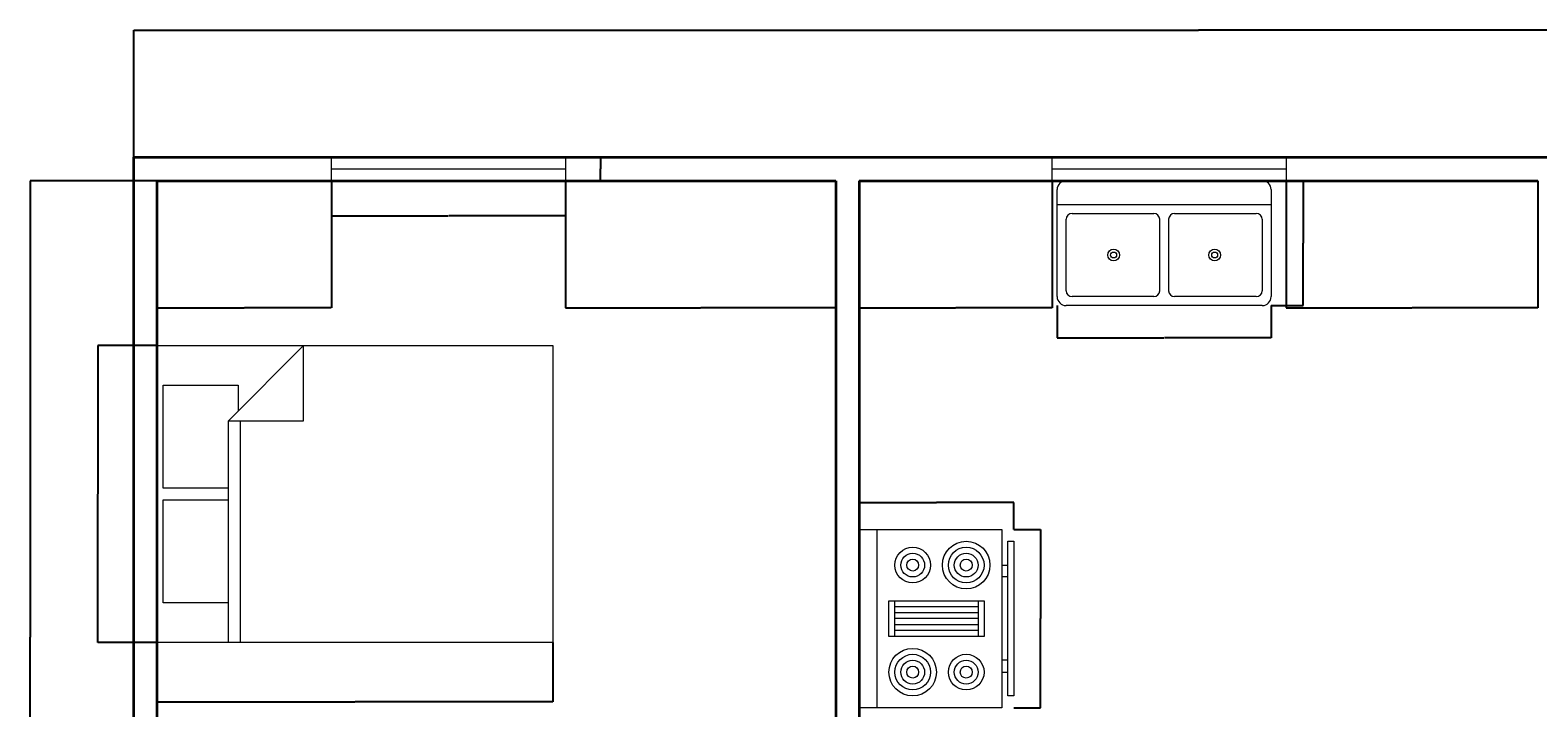
# Model space of a CAD drawing. Units: millimetres. Extents: x 1426 to 11512, y -8522 to 2664.
# Tile 3 of 4: x 1426 to 7869, y -230 to 2664. Entities that reach past the tile are written whole.
import ezdxf

# ---------------------------------------------------------------- set-up
doc = ezdxf.new("R2010")
doc.units = ezdxf.units.MM
for name, color, linetype, lineweight in [('A-ANNO-DIMS', 2, 'Continuous', 18), ('A-EQPM', 8, 'Continuous', 20), ('A-FLOR-FIXT', 9, 'Continuous', 20), ('A-FURN', 8, 'Continuous', 18), ('A-GLAZ', 4, 'Continuous', 18), ('A-WALL', 7, 'Continuous', 35)]:
    doc.layers.add(name, color=color, linetype=linetype, lineweight=lineweight)
doc.styles.get("Standard").update_dxf_attribs({"font": 'arial.ttf'})
doc.dimstyles.get("Standard").update_dxf_attribs({"dimtxt": 0.18, "dimasz": 0.18, "dimexe": 0.18, "dimexo": 0.0625, "dimgap": 0.09, "dimtad": 0, "dimtih": 1, "dimtoh": 1, "dimdec": 4, "dimzin": 0, "dimdsep": 46, "dimtxsty": 'Standard', "dimcen": 0.09, "dimadec": 0, "dimazin": 0, "dimtfac": 1, "dimtdec": 4, "dimtofl": 0, "dimtmove": 0, "dimatfit": 3, "dimfxl": 1, "dimtolj": 1, "dimtzin": 0, "dimarcsym": 0})

# ---------------------------------------------------------------- blocks, each defined once
blk = doc.blocks.new('Range-Oven - 30 in top')
for p, q in [((0, -3), (30, -3)), ((12, -6), (18, -6)), ((13, -20), (13, -6)), ((14, -6), (14, -20)), ((15, -20), (15, -6)), ((16, -6), (16, -20)), ((17, -20), (17, -6)), ((18, -20), (12, -20)), ((6, -24), (6, -25)), ((8, -25), (8, -24)), ((22, -25), (22, -24)), ((24, -24), (24, -25))]:
    blk.add_line(p, q)
for points in [[(0, -24), (0, 0), (30, 0), (30, -24)], [(12, -21), (12, -5), (18, -5), (18, -21)], [(2, -26), (2, -25), (28, -25), (28, -26)]]:
    blk.add_lwpolyline(points, close=True)
for centre, radius in [((6, -9), 4), ((6, -9), 3), ((6, -9), 2), ((24, -9), 3), ((24, -9), 2), ((6, -9), 1), ((24, -9), 1), ((6, -18), 3), ((24, -18), 4), ((24, -18), 3), ((6, -18), 2), ((6, -18), 1), ((24, -18), 2), ((24, -18), 1)]:
    blk.add_circle(centre, radius)
blk = doc.blocks.new('Sink-double - 36 in top')
for p, q in [((-18, -4), (18, -4)), ((-0.75, -18.5), (-0.75, -6.5)), ((0.75, -6.5), (0.75, -18.5))]:
    blk.add_line(p, q)
for points in [[(-16.5, 0), (16.5, 0)], [(-18, -19.5), (-18, -1.5)], [(18, -1.5), (18, -19.5)], [(-16.5, -18.5), (-16.5, -6.5)], [(-15.5, -5.5), (-1.75, -5.5)], [(1.75, -5.5), (15.5, -5.5)], [(16.5, -6.5), (16.5, -18.5)], [(-1.75, -19.5), (-15.5, -19.5)], [(15.5, -19.5), (1.75, -19.5)], [(16.5, -21), (-16.5, -21)]]:
    blk.add_lwpolyline(points)
for centre, radius in [((-8.5, -12.5), 1), ((-8.5, -12.5), 0.5), ((8.5, -12.5), 1), ((8.5, -12.5), 0.5)]:
    blk.add_circle(centre, radius)
for centre, radius, start, end in [((-16.5, -1.5), 1.5, 90, 180), ((16.5, -1.5), 1.5, 0, 90), ((-15.5, -6.5), 1, 90, 180), ((-1.75, -6.5), 1, 0, 90), ((1.75, -6.5), 1, 90, 180), ((15.5, -6.5), 1, 0, 90), ((-16.5, -19.5), 1.5, 180, 270), ((-15.5, -18.5), 1, 180, 270), ((-1.75, -18.5), 1, 270, 0), ((1.75, -18.5), 1, 180, 270), ((15.5, -18.5), 1, 270, 0), ((16.5, -19.5), 1.5, 270, 0)]:
    blk.add_arc(centre, radius, start, end)
blk = doc.blocks.new('Bed - Queen')
for p, q in [((0, -80.00003), (0, 0)), ((0, 0), (59.99999, 0)), ((59.99999, 0), (59.99999, -80.00003)), ((7.99999, -1.2), (28.79998, -1.2)), ((7.99999, -14.4), (7.99999, -1.2)), ((28.79998, -1.2), (28.79998, -14.4)), ((31.19999, -1.2), (51.99999, -1.2)), ((31.19999, -14.4), (31.19999, -1.2)), ((51.99999, -1.2), (51.99999, -16.4)), ((0, -14.4), (44.8, -14.4)), ((59.99999, -29.6), (44.8, -14.4)), ((44.8, -14.4), (44.8, -29.6)), ((44.8, -16.8), (0, -16.8)), ((51.99999, -16.4), (46.79936, -16.4)), ((44.8, -29.6), (59.99999, -29.6)), ((59.99999, -80.00003), (0, -80.00003))]:
    blk.add_line(p, q)
blk = doc.blocks.new('WIN-1000')
for p, q in [((0, 100), (1000, 100)), ((0, 0), (0, 100)), ((1000, 100), (1000, 0)), ((0, 50), (1000, 50)), ((1000, 0), (0, 0))]:
    blk.add_line(p, q)
blk = doc.blocks.new('*D14')
at = {"layer": 'A-ANNO-DIMS', "color": 0, "lineweight": -2, "transparency": 16777216}
for p, q in [((2713.3, 2020.9), (2713.3, 1870.8)), ((3713.3, 2020.9), (3713.3, 1870.8)), ((2713.5, 1870.9), (3212.1, 1870.9)), ((3713.1, 1870.9), (3214.6, 1870.9))]:
    blk.add_line(p, q, dxfattribs=at)
at = {"layer": 'A-ANNO-DIMS', "color": 0, "transparency": 16777216}
for points in [[(2713.5, 1871), (2713.5, 1870.9), (2713.3, 1870.9)], [(3713.1, 1871), (3713.1, 1870.9), (3713.3, 1870.9)]]:
    blk.add_solid(points, dxfattribs=at)
at = {"layer": 'Defpoints', "color": 0, "transparency": 16777216}
for p in [(2713.3, 2020.9), (3713.3, 2020.9), (3713.3, 1870.9)]:
    blk.add_point(p, dxfattribs=at)
at = {"layer": 'A-ANNO-DIMS', "color": 0, "transparency": 16777216, "insert": (3213.3, 1870.9), "char_height": 0.18, "attachment_point": 5}
blk.add_mtext('\\A1;WINDOW 1000 TYP.', dxfattribs=at)
blk = doc.blocks.new('*D15')
at = {"layer": 'A-ANNO-DIMS', "color": 0, "lineweight": -2, "transparency": 16777216}
for p, q in [((3713.4, 2120.9), (3863.5, 2120.9)), ((3863.3, 2120.8), (3863.3, 2071.1)), ((3863.3, 2021.1), (3863.3, 2070.8)), ((3713.4, 2020.9), (3863.5, 2020.9))]:
    blk.add_line(p, q, dxfattribs=at)
at = {"layer": 'A-ANNO-DIMS', "color": 0, "transparency": 16777216}
for points in [[(3863.3, 2120.8), (3863.3, 2120.8), (3863.3, 2120.9)], [(3863.3, 2021.1), (3863.3, 2021.1), (3863.3, 2020.9)]]:
    blk.add_solid(points, dxfattribs=at)
at = {"layer": 'Defpoints', "color": 0, "transparency": 16777216}
for p in [(3713.3, 2120.9), (3863.3, 2120.9), (3713.3, 2020.9)]:
    blk.add_point(p, dxfattribs=at)
at = {"layer": 'A-ANNO-DIMS', "color": 0, "transparency": 16777216, "insert": (3863.3, 2070.9), "char_height": 0.18, "attachment_point": 5}
blk.add_mtext('\\A1;100 TYP.', dxfattribs=at)
blk = doc.blocks.new('*D22')
at = {"layer": 'A-ANNO-DIMS', "color": 0, "lineweight": -2, "transparency": 16777216}
for p, q in [((1968.9, 49), (1968.9, -204.6)), ((3659.2, 49), (3659.2, -204.6)), ((1969.1, -204.5), (2813.4, -204.5)), ((3659, -204.5), (2814.7, -204.5))]:
    blk.add_line(p, q, dxfattribs=at)
at = {"layer": 'A-ANNO-DIMS', "color": 0, "transparency": 16777216}
for points in [[(1969.1, -204.4), (1969.1, -204.5), (1968.9, -204.5)], [(3659, -204.4), (3659, -204.5), (3659.2, -204.5)]]:
    blk.add_solid(points, dxfattribs=at)
at = {"layer": 'Defpoints', "color": 0, "transparency": 16777216}
for p in [(1968.9, 49.1), (3659.2, 49.1), (1968.9, -204.5)]:
    blk.add_point(p, dxfattribs=at)
at = {"layer": 'A-ANNO-DIMS', "color": 0, "transparency": 16777216, "insert": (2814, -204.5), "char_height": 0.18, "attachment_point": 5}
blk.add_mtext('\\A1;BED 1690', dxfattribs=at)
blk = doc.blocks.new('*D23')
at = {"layer": 'A-ANNO-DIMS', "color": 0, "lineweight": -2, "transparency": 16777216}
for p, q in [((1968.8, 1316.9), (1715.1, 1316.9)), ((1715.3, 1316.7), (1715.3, 683.2)), ((1715.3, 49.3), (1715.3, 682.8)), ((1968.8, 49.1), (1715.1, 49.1))]:
    blk.add_line(p, q, dxfattribs=at)
at = {"layer": 'A-ANNO-DIMS', "color": 0, "transparency": 16777216}
for points in [[(1715.3, 1316.7), (1715.3, 1316.7), (1715.3, 1316.9)], [(1715.3, 49.3), (1715.3, 49.3), (1715.3, 49.1)]]:
    blk.add_solid(points, dxfattribs=at)
at = {"layer": 'Defpoints', "color": 0, "transparency": 16777216}
for p in [(1715.3, 1316.9), (1968.9, 1316.9), (1968.9, 49.1)]:
    blk.add_point(p, dxfattribs=at)
at = {"layer": 'A-ANNO-DIMS', "color": 0, "transparency": 16777216, "insert": (1715.3, 683), "char_height": 0.18, "attachment_point": 5}
blk.add_mtext('\\A1;1268', dxfattribs=at)
blk = doc.blocks.new('*D28')
at = {"layer": 'A-ANNO-DIMS', "color": 0, "lineweight": -2, "transparency": 16777216}
for p, q in [((5629.3, 531.7), (5743.8, 531.7)), ((5743.6, 531.5), (5743.6, 150.9)), ((5743.6, -230.1), (5743.6, 150.5)), ((5629.3, -230.3), (5743.8, -230.3))]:
    blk.add_line(p, q, dxfattribs=at)
at = {"layer": 'A-ANNO-DIMS', "color": 0, "transparency": 16777216}
for points in [[(5743.5, 531.5), (5743.6, 531.5), (5743.6, 531.7)], [(5743.5, -230.1), (5743.6, -230.1), (5743.6, -230.3)]]:
    blk.add_solid(points, dxfattribs=at)
at = {"layer": 'Defpoints', "color": 0, "transparency": 16777216}
for p in [(5629.3, 531.7), (5743.6, 531.7), (5629.3, -230.3)]:
    blk.add_point(p, dxfattribs=at)
at = {"layer": 'A-ANNO-DIMS', "color": 0, "transparency": 16777216, "insert": (5743.6, 150.7), "char_height": 0.18, "attachment_point": 5}
blk.add_mtext('\\A1;RANGE 762', dxfattribs=at)
blk = doc.blocks.new('*D29')
at = {"layer": 'A-ANNO-DIMS', "color": 0, "lineweight": -2, "transparency": 16777216}
for p, q in [((4968.9, 531.8), (4968.9, 646.2)), ((4969.1, 646), (5298.8, 646)), ((5629.1, 646), (5299.4, 646)), ((5629.3, 531.8), (5629.3, 646.2))]:
    blk.add_line(p, q, dxfattribs=at)
at = {"layer": 'A-ANNO-DIMS', "color": 0, "transparency": 16777216}
for points in [[(4969.1, 646), (4969.1, 646), (4968.9, 646)], [(5629.1, 646), (5629.1, 646), (5629.3, 646)]]:
    blk.add_solid(points, dxfattribs=at)
at = {"layer": 'Defpoints', "color": 0, "transparency": 16777216}
for p in [(4968.9, 646), (4968.9, 531.7), (5629.3, 531.7)]:
    blk.add_point(p, dxfattribs=at)
at = {"layer": 'A-ANNO-DIMS', "color": 0, "transparency": 16777216, "insert": (5299.1, 646), "char_height": 0.18, "attachment_point": 5}
blk.add_mtext('\\A1;660', dxfattribs=at)
blk = doc.blocks.new('*D30')
at = {"layer": 'A-ANNO-DIMS', "color": 0, "lineweight": -2, "transparency": 16777216}
for p, q in [((5814.7, 1487.5), (5814.7, 1350.2)), ((6729.1, 1487.5), (6729.1, 1350.2)), ((5814.9, 1350.4), (6270.7, 1350.4)), ((6729, 1350.4), (6273.1, 1350.4))]:
    blk.add_line(p, q, dxfattribs=at)
at = {"layer": 'A-ANNO-DIMS', "color": 0, "transparency": 16777216}
for points in [[(5814.9, 1350.4), (5814.9, 1350.4), (5814.7, 1350.4)], [(6729, 1350.4), (6729, 1350.4), (6729.1, 1350.4)]]:
    blk.add_solid(points, dxfattribs=at)
at = {"layer": 'Defpoints', "color": 0, "transparency": 16777216}
for p in [(5814.7, 1487.5), (6729.1, 1487.5), (6729.1, 1350.4)]:
    blk.add_point(p, dxfattribs=at)
at = {"layer": 'A-ANNO-DIMS', "color": 0, "transparency": 16777216, "insert": (6271.9, 1350.4), "char_height": 0.18, "attachment_point": 5}
blk.add_mtext('\\A1;KITCHEN SINK 914', dxfattribs=at)
blk = doc.blocks.new('*D31')
at = {"layer": 'A-ANNO-DIMS', "color": 0, "lineweight": -2, "transparency": 16777216}
for p, q in [((6729.2, 2020.9), (6866.5, 2020.9)), ((6866.3, 2020.8), (6866.3, 1754.4)), ((6866.3, 1487.7), (6866.3, 1754.1)), ((6729.2, 1487.5), (6866.5, 1487.5))]:
    blk.add_line(p, q, dxfattribs=at)
at = {"layer": 'A-ANNO-DIMS', "color": 0, "transparency": 16777216}
for points in [[(6866.3, 2020.8), (6866.3, 2020.8), (6866.3, 2020.9)], [(6866.3, 1487.7), (6866.3, 1487.7), (6866.3, 1487.5)]]:
    blk.add_solid(points, dxfattribs=at)
at = {"layer": 'Defpoints', "color": 0, "transparency": 16777216}
for p in [(6729.1, 2020.9), (6866.3, 2020.9), (6729.1, 1487.5)]:
    blk.add_point(p, dxfattribs=at)
at = {"layer": 'A-ANNO-DIMS', "color": 0, "transparency": 16777216, "insert": (6866.3, 1754.2), "char_height": 0.18, "attachment_point": 5}
blk.add_mtext('\\A1;533', dxfattribs=at)
blk = doc.blocks.new('*D39')
at = {"layer": 'A-ANNO-DIMS', "color": 0, "lineweight": -2, "transparency": 16777216}
for p, q in [((1868.9, 2121), (1868.9, 2663.6)), ((1869.1, 2663.4), (6418.5, 2663.4)), ((10968.7, 2663.4), (6419.2, 2663.4)), ((10968.9, 2121), (10968.9, 2663.6))]:
    blk.add_line(p, q, dxfattribs=at)
at = {"layer": 'A-ANNO-DIMS', "color": 0, "transparency": 16777216}
for points in [[(1869.1, 2663.5), (1869.1, 2663.4), (1868.9, 2663.4)], [(10968.7, 2663.5), (10968.7, 2663.4), (10968.9, 2663.4)]]:
    blk.add_solid(points, dxfattribs=at)
at = {"layer": 'Defpoints', "color": 0, "transparency": 16777216}
for p in [(10968.9, 2663.4), (1868.9, 2120.9), (10968.9, 2120.9)]:
    blk.add_point(p, dxfattribs=at)
at = {"layer": 'A-ANNO-DIMS', "color": 0, "transparency": 16777216, "insert": (6418.9, 2663.4), "char_height": 0.18, "attachment_point": 5}
blk.add_mtext('\\A1;9100', dxfattribs=at)
blk = doc.blocks.new('*D43')
at = {"layer": 'A-ANNO-DIMS', "color": 0, "lineweight": -2, "transparency": 16777216}
for p, q in [((1968.8, 2020.9), (1426.2, 2020.9)), ((1426.4, 2020.8), (1426.4, 71.1)), ((1426.4, -1878.9), (1426.4, 70.8)), ((1968.8, -1879.1), (1426.2, -1879.1))]:
    blk.add_line(p, q, dxfattribs=at)
at = {"layer": 'A-ANNO-DIMS', "color": 0, "transparency": 16777216}
for points in [[(1426.3, 2020.8), (1426.4, 2020.8), (1426.4, 2020.9)], [(1426.3, -1878.9), (1426.4, -1878.9), (1426.4, -1879.1)]]:
    blk.add_solid(points, dxfattribs=at)
at = {"layer": 'Defpoints', "color": 0, "transparency": 16777216}
for p in [(1426.4, 2020.9), (1968.9, 2020.9), (1968.9, -1879.1)]:
    blk.add_point(p, dxfattribs=at)
at = {"layer": 'A-ANNO-DIMS', "color": 0, "transparency": 16777216, "insert": (1426.4, 70.9), "char_height": 0.18, "attachment_point": 5}
blk.add_mtext('\\A1;3900', dxfattribs=at)
blk = doc.blocks.new('*D54')
at = {"layer": 'A-ANNO-DIMS', "color": 0, "lineweight": -2, "transparency": 16777216}
for p, q in [((1968.9, 2020.9), (1968.9, 1478.3)), ((2713.3, 2020.9), (2713.3, 1478.3)), ((1969.1, 1478.4), (2340.7, 1478.4)), ((2713.1, 1478.4), (2341.5, 1478.4))]:
    blk.add_line(p, q, dxfattribs=at)
at = {"layer": 'A-ANNO-DIMS', "color": 0, "transparency": 16777216}
for points in [[(1969.1, 1478.5), (1969.1, 1478.4), (1968.9, 1478.4)], [(2713.1, 1478.5), (2713.1, 1478.4), (2713.3, 1478.4)]]:
    blk.add_solid(points, dxfattribs=at)
at = {"layer": 'Defpoints', "color": 0, "transparency": 16777216}
for p in [(1968.9, 2020.9), (2713.3, 2020.9), (1968.9, 1478.4)]:
    blk.add_point(p, dxfattribs=at)
at = {"layer": 'A-ANNO-DIMS', "color": 0, "transparency": 16777216, "insert": (2341.1, 1478.4), "char_height": 0.18, "attachment_point": 5}
blk.add_mtext('\\A1;744.4', dxfattribs=at)
blk = doc.blocks.new('*D55')
at = {"layer": 'A-ANNO-DIMS', "color": 0, "lineweight": -2, "transparency": 16777216}
for p, q in [((3713.3, 2020.9), (3713.3, 1478.3)), ((4868.9, 2020.9), (4868.9, 1478.3)), ((3713.5, 1478.4), (4290.6, 1478.4)), ((4868.7, 1478.4), (4291.5, 1478.4))]:
    blk.add_line(p, q, dxfattribs=at)
at = {"layer": 'A-ANNO-DIMS', "color": 0, "transparency": 16777216}
for points in [[(3713.5, 1478.5), (3713.5, 1478.4), (3713.3, 1478.4)], [(4868.7, 1478.5), (4868.7, 1478.4), (4868.9, 1478.4)]]:
    blk.add_solid(points, dxfattribs=at)
at = {"layer": 'Defpoints', "color": 0, "transparency": 16777216}
for p in [(3713.3, 2020.9), (4868.9, 2020.9), (3713.3, 1478.4)]:
    blk.add_point(p, dxfattribs=at)
at = {"layer": 'A-ANNO-DIMS', "color": 0, "transparency": 16777216, "insert": (4291.1, 1478.4), "char_height": 0.18, "attachment_point": 5}
blk.add_mtext('\\A1;1155.6', dxfattribs=at)
blk = doc.blocks.new('*D56')
at = {"layer": 'A-ANNO-DIMS', "color": 0, "lineweight": -2, "transparency": 16777216}
for p, q in [((4968.9, 2020.9), (4968.9, 1478.3)), ((5793.2, 2020.9), (5793.2, 1478.3)), ((4969.1, 1478.4), (5380.6, 1478.4)), ((5793, 1478.4), (5381.4, 1478.4))]:
    blk.add_line(p, q, dxfattribs=at)
at = {"layer": 'A-ANNO-DIMS', "color": 0, "transparency": 16777216}
for points in [[(4969.1, 1478.5), (4969.1, 1478.4), (4968.9, 1478.4)], [(5793, 1478.5), (5793, 1478.4), (5793.2, 1478.4)]]:
    blk.add_solid(points, dxfattribs=at)
at = {"layer": 'Defpoints', "color": 0, "transparency": 16777216}
for p in [(4968.9, 2020.9), (5793.2, 2020.9), (4968.9, 1478.4)]:
    blk.add_point(p, dxfattribs=at)
at = {"layer": 'A-ANNO-DIMS', "color": 0, "transparency": 16777216, "insert": (5381, 1478.4), "char_height": 0.18, "attachment_point": 5}
blk.add_mtext('\\A1;824.3', dxfattribs=at)
blk = doc.blocks.new('*D57')
at = {"layer": 'A-ANNO-DIMS', "color": 0, "lineweight": -2, "transparency": 16777216}
for p, q in [((6793.2, 2020.9), (6793.2, 1478.3)), ((7868.9, 2020.9), (7868.9, 1478.3)), ((6793.4, 1478.4), (7330.6, 1478.4)), ((7868.7, 1478.4), (7331.5, 1478.4))]:
    blk.add_line(p, q, dxfattribs=at)
at = {"layer": 'A-ANNO-DIMS', "color": 0, "transparency": 16777216}
for points in [[(6793.4, 1478.5), (6793.4, 1478.4), (6793.2, 1478.4)], [(7868.7, 1478.5), (7868.7, 1478.4), (7868.9, 1478.4)]]:
    blk.add_solid(points, dxfattribs=at)
at = {"layer": 'Defpoints', "color": 0, "transparency": 16777216}
for p in [(6793.2, 2020.9), (7868.9, 2020.9), (6793.2, 1478.4)]:
    blk.add_point(p, dxfattribs=at)
at = {"layer": 'A-ANNO-DIMS', "color": 0, "transparency": 16777216, "insert": (7331, 1478.4), "char_height": 0.18, "attachment_point": 5}
blk.add_mtext('\\A1;1075.7', dxfattribs=at)

msp = doc.modelspace()

# ---------------------------------------------------------------- linework, layer by layer
at = {"layer": 'A-WALL'}
for p, q in [((1868.87, 2120.94), (8976.97, 2120.94)), ((1868.87, -7979.06), (1868.87, 2120.94)), ((1968.87, 2020.94), (4868.87, 2020.94)), ((1968.87, -1879.06), (1968.87, 2020.94)), ((4868.87, 2020.94), (4868.87, -1879.06)), ((4968.87, 2020.94), (4968.87, -1879.06)), ((4968.87, 2020.94), (7868.87, 2020.94))]:
    msp.add_line(p, q, dxfattribs=at)

# ---------------------------------------------------------------- block references
at = {"layer": 'A-EQPM', "xscale": 25.4, "yscale": 25.4, "zscale": 25.4, "rotation": 90}
msp.add_blockref('Range-Oven - 30 in top', (4968.87, -230.3), dxfattribs=at)
at = {"layer": 'A-FLOR-FIXT', "xscale": 25.4, "yscale": 25.4, "zscale": 25.4}
msp.add_blockref('Sink-double - 36 in top', (6271.93, 2020.94), dxfattribs=at)
at = {"layer": 'A-FURN', "xscale": 21.12936966835213, "yscale": 21.12936966835213, "zscale": 21.12936966835213, "rotation": 89.99999999999999}
msp.add_blockref('Bed - Queen', (1968.87, 49.09), dxfattribs=at)
at = {"layer": 'A-GLAZ'}
for p in [(2713.31, 2020.94), (5793.19, 2020.94)]:
    msp.add_blockref('WIN-1000', p, dxfattribs=at)

# ---------------------------------------------------------------- dimensions: what is measured, and where the dimension line sits
at = {"layer": 'A-ANNO-DIMS'}
dim = msp.add_linear_dim(base=(10968.87, 2663.44), p1=(1868.87, 2120.94), p2=(10968.87, 2120.94), dimstyle='Standard', override={"dimdec": 0, "dimlfac": 1, "dimrnd": 0, "dimzin": 0, "dimdsep": 46, "dimlunit": 2}, dxfattribs=at)
dim.commit()
dim.dimension.update_dxf_attribs({"geometry": '*D39', "text_midpoint": (6418.87, 2663.44)})
for base, p1, p2, angle, text, picture, middle in [((3863.31, 2120.94), (3713.31, 2020.94), (3713.31, 2120.94), 90, '<> TYP.', '*D15', (3863.31, 2070.94)), ((5743.57, 531.7), (5629.27, -230.3), (5629.27, 531.7), 90, 'RANGE <>', '*D28', (5743.57, 150.7)), ((1968.87, -204.46), (3659.22, 49.09), (1968.87, 49.09), 180, 'BED <>', '*D22', (2814.05, -204.46))]:
    dim = msp.add_linear_dim(base=base, p1=p1, p2=p2, angle=angle, text=text, dimstyle='Standard', override={"dimdec": 0, "dimlfac": 1, "dimrnd": 0, "dimzin": 0, "dimdsep": 46, "dimlunit": 2}, dxfattribs=at)
    dim.commit()
    dim.dimension.update_dxf_attribs({"geometry": picture, "text_midpoint": middle})
for base, p1, p2, angle, override, picture, middle in [((1426.37, 2020.94), (1968.87, -1879.06), (1968.87, 2020.94), 90, {"dimdec": 0, "dimlfac": 1, "dimrnd": 0, "dimzin": 0, "dimdsep": 46, "dimlunit": 2}, '*D43', (1426.37, 70.94)), ((1968.87, 1478.44), (2713.31, 2020.94), (1968.87, 2020.94), 180, {"dimdec": 1, "dimlfac": 1, "dimrnd": 0, "dimzin": 0, "dimdsep": 46, "dimlunit": 2}, '*D54', (2341.09, 1478.44)), ((3713.31, 1478.44), (4868.87, 2020.94), (3713.31, 2020.94), 180, {"dimdec": 1, "dimlfac": 1, "dimrnd": 0, "dimzin": 0, "dimdsep": 46, "dimlunit": 2}, '*D55', (4291.09, 1478.44)), ((4968.87, 1478.44), (5793.19, 2020.94), (4968.87, 2020.94), 180, {"dimdec": 1, "dimlfac": 1, "dimrnd": 0, "dimzin": 0, "dimdsep": 46, "dimlunit": 2}, '*D56', (5381.03, 1478.44)), ((6866.29, 2020.94), (6729.13, 1487.54), (6729.13, 2020.94), 90, {"dimdec": 0, "dimlfac": 1, "dimrnd": 0, "dimzin": 0, "dimdsep": 46, "dimlunit": 2}, '*D31', (6866.29, 1754.24)), ((6793.19, 1478.44), (7868.87, 2020.94), (6793.19, 2020.94), 180, {"dimdec": 1, "dimlfac": 1, "dimrnd": 0, "dimzin": 0, "dimdsep": 46, "dimlunit": 2}, '*D57', (7331.03, 1478.44)), ((1715.32, 1316.86), (1968.87, 49.09), (1968.87, 1316.86), 90, {"dimdec": 0, "dimlfac": 1, "dimrnd": 0, "dimzin": 0, "dimdsep": 46, "dimlunit": 2}, '*D23', (1715.32, 682.98)), ((4968.87, 646), (5629.27, 531.7), (4968.87, 531.7), 180, {"dimdec": 0, "dimlfac": 1, "dimrnd": 0, "dimzin": 0, "dimdsep": 46, "dimlunit": 2}, '*D29', (5299.07, 646))]:
    dim = msp.add_linear_dim(base=base, p1=p1, p2=p2, angle=angle, dimstyle='Standard', override=override, dxfattribs=at)
    dim.commit()
    dim.dimension.update_dxf_attribs({"geometry": picture, "text_midpoint": middle})
for base, p1, p2, text, picture, middle in [((3713.31, 1870.94), (2713.31, 2020.94), (3713.31, 2020.94), 'WINDOW <> TYP.', '*D14', (3213.31, 1870.94)), ((6729.13, 1350.38), (5814.73, 1487.54), (6729.13, 1487.54), 'KITCHEN SINK <>', '*D30', (6271.93, 1350.38))]:
    dim = msp.add_linear_dim(base=base, p1=p1, p2=p2, text=text, dimstyle='Standard', override={"dimdec": 0, "dimlfac": 1, "dimrnd": 0, "dimzin": 0, "dimdsep": 46, "dimlunit": 2}, dxfattribs=at)
    dim.commit()
    dim.dimension.update_dxf_attribs({"geometry": picture, "text_midpoint": middle})

doc.saveas('drawing.dxf')
